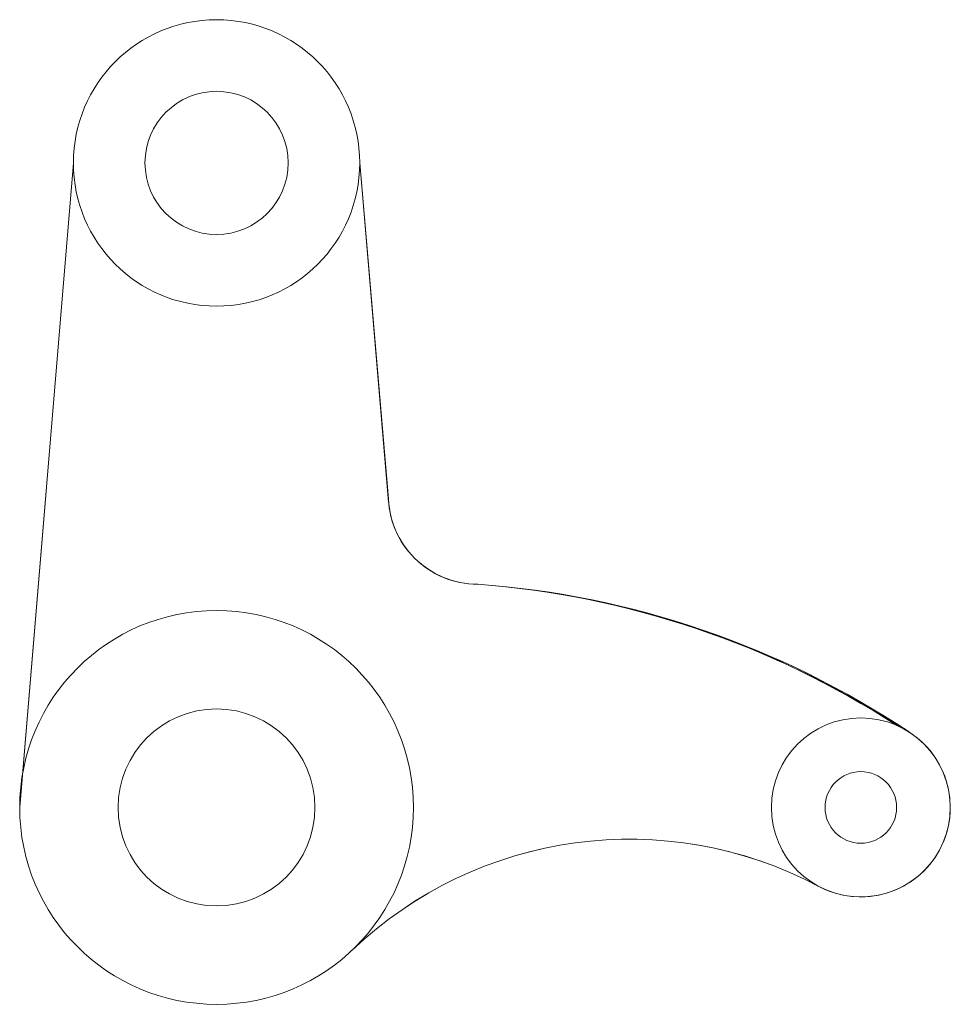
# Model space of a CAD drawing. Units: millimetres. Extents: x 3903 to 4007, y 1540 to 1650.
import ezdxf

# ---------------------------------------------------------------- set-up
doc = ezdxf.new("R2010")
doc.units = ezdxf.units.MM
doc.layers.add('M-CONS', color=8, linetype='Continuous', lineweight=18)

msp = doc.modelspace()

# ---------------------------------------------------------------- linework, layer by layer
at = {"layer": 'M-CONS'}
for p, q in [((3903.11, 1561.61), (3909.11, 1633.61)), ((3903.11, 1561.61, 27.51), (3909.11, 1633.61, 27.51))]:
    msp.add_line(p, q, dxfattribs=at)
for points, elevation in [([(3903.41, 1565.25), (3909.11, 1633.61, -1), (3941.11, 1633.61), (3944.34, 1595.7)], 38), ([(4001.13, 1570.77, 0.12548), (3954.3, 1586.54, -0.414214), (3944.3, 1596.54), (3941.11, 1633.61)], 27.51), ([(3940.27, 1545.67, -0.322846), (3992.41, 1552.79, 1.038417), (4001.13, 1570.77)], 38)]:
    msp.add_lwpolyline(points, format="xyb", dxfattribs=dict(at, elevation=elevation))
msp.add_lwpolyline([(4001.13, 1570.77, 0.12548), (3954.3, 1586.54, -0.414214), (3944.3, 1596.54), (3941.11, 1633.61)], format="xyb", dxfattribs=at)
for centre, radius in [((3925.11, 1633.61), 16), ((3925.11, 1633.61, 27.51), 16), ((3925.11, 1633.61), 8), ((3925.11, 1633.61, 38), 8), ((3925.11, 1633.61, 27.51), 8), ((3925.11, 1561.61), 22), ((3925.11, 1561.61, 38), 22), ((3925.11, 1561.61, 38), 22), ((3925.11, 1561.61, 27.51), 22), ((3925.11, 1561.61), 11), ((3925.11, 1561.61, 38), 11), ((3925.11, 1561.61, 38), 11), ((3925.11, 1561.61, 27.51), 11), ((3997.11, 1561.61), 10), ((3997.11, 1561.61, 27.51), 10), ((3997.11, 1561.61), 4), ((3997.11, 1561.61), 4), ((3997.11, 1561.61, 38), 4), ((3997.11, 1561.61, 27.51), 4), ((3997.11, 1561.61, 27.51), 4)]:
    msp.add_circle(centre, radius, dxfattribs=at)
for centre, radius, start, end in [((3954.3, 1596.54, 38), 10, 180, 270), ((3946.86, 1486.82), 100, 56.9853, 85.7311), ((3947.07, 1486.81, 38), 100, 56.3426, 85.8533), ((3946.86, 1486.82, 27.51), 100, 56.9853, 85.7311), ((3971.28, 1513.06), 45, 61.9854, 133.5553), ((3971.28, 1513.06, 27.51), 45, 61.9854, 133.5553)]:
    msp.add_arc(centre, radius, start, end, dxfattribs=at)

doc.saveas('drawing.dxf')
